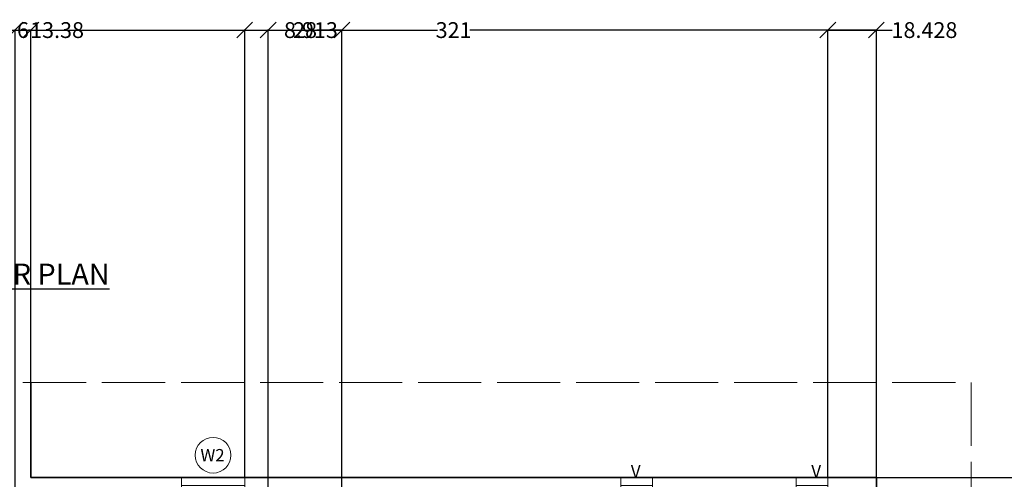
# Model space of a CAD drawing. Units: inches. Extents: x -1198 to -69, y -512 to 437.
# Tile 49 of 50: x -696 to -322, y 263 to 437. Entities that reach past the tile are written whole.
import ezdxf

# ---------------------------------------------------------------- set-up
doc = ezdxf.new("R2010")
doc.units = ezdxf.units.IN
doc.header["$MEASUREMENT"] = 0
doc.linetypes.add('ACAD_ISO02W100', pattern=[15, 12, -3])
for name, color, linetype, lineweight in [('A-ANNO-DIMS', 2, 'Continuous', 18), ('A-ANNO-SYMB', 7, 'Continuous', 18), ('A-ANNO-TEXT', 7, 'Continuous', 25), ('A-WALL', 7, 'Continuous', 35), ('C-PROP', 141, 'ACAD_ISO02W100', 18), ('Doors', 140, 'Continuous', 25), ('windows', 160, 'Continuous', 18)]:
    doc.layers.add(name, color=color, linetype=linetype, lineweight=lineweight)
doc.styles.get("Standard").update_dxf_attribs({"font": 'arial.ttf'})
doc.dimstyles.get("Standard").update_dxf_attribs({"dimtxt": 6, "dimasz": 6, "dimexe": 0.18, "dimexo": 0.0625, "dimgap": 0.09, "dimtad": 0, "dimtih": 1, "dimtoh": 1, "dimdec": 0, "dimzin": 0, "dimdsep": 46, "dimlunit": 4, "dimtxsty": 'Standard', "dimblk": 'OBLIQUE', "dimcen": 0.09, "dimadec": 0, "dimazin": 0, "dimtfac": 1, "dimtdec": 0, "dimtofl": 0, "dimtmove": 0, "dimatfit": 3, "dimfxl": 1, "dimtolj": 1, "dimtzin": 0, "dimarcsym": 0})

# ---------------------------------------------------------------- blocks, each defined once
blk = doc.blocks.new('*U4')
for p, q in [((0, 0), (0, -6)), ((28, 0), (28, -6))]:
    blk.add_line(p, q)
blk.add_lwpolyline([(0, 0), (0, 28), (1.75, 28), (1.75, 0)], close=True)
blk.add_arc((0, 0), 28, 0, 90)
blk = doc.blocks.new('WIN-W2-24')
at = {"ltscale": 10}
for p, q in [((0, 6), (0, 0)), ((24, 6), (24, 0)), ((0, 3), (24, 3))]:
    blk.add_line(p, q, dxfattribs=at)
blk = doc.blocks.new('VENT-12')
at = {"ltscale": 10}
for p, q in [((0, 6), (0, 0)), ((12, 6), (12, 0)), ((0, 3), (12, 3))]:
    blk.add_line(p, q, dxfattribs=at)
blk = doc.blocks.new('TAG-W2')
at = {"ltscale": 10}
blk.add_circle((0, 0), 6.77, dxfattribs=at)
blk.add_text('W2', height=4.7, dxfattribs=at).set_placement((-4.79, -2.36))
blk = doc.blocks.new('_Oblique')
at = {"color": 0, "linetype": 'ByBlock', "lineweight": -2}
blk.add_line((-0.5, -0.5), (0.5, 0.5), dxfattribs=at)
blk = doc.blocks.new('*D63')
at = {"layer": 'A-ANNO-DIMS', "color": 0, "lineweight": -2, "ltscale": 10, "transparency": 16777216}
for p, q in [((-370.69, 263.23), (-79.37, 263.23)), ((-79.55, 263.23), (-79.55, 20.38)), ((-79.55, -228.77), (-79.55, 14.07)), ((-370.69, -228.77), (-79.37, -228.77))]:
    blk.add_line(p, q, dxfattribs=at)
at = {"layer": 'DEFPOINTS', "color": 0, "ltscale": 10, "transparency": 16777216}
for p in [(-370.75, 263.23), (-79.55, 263.23), (-370.75, -228.77)]:
    blk.add_point(p, dxfattribs=at)
at = {"layer": 'A-ANNO-DIMS', "color": 0, "lineweight": -2, "ltscale": 10, "transparency": 16777216, "xscale": 6, "yscale": 6, "zscale": 6}
for p, rotation in [((-79.55, 263.23), 90), ((-79.55, -228.77), 270)]:
    blk.add_blockref('_Oblique', p, dxfattribs=dict(at, rotation=rotation))
at = {"layer": 'A-ANNO-DIMS', "color": 0, "ltscale": 10, "transparency": 16777216, "insert": (-79.55, 17.23), "char_height": 6, "attachment_point": 5}
blk.add_mtext('\\A1;492', dxfattribs=at)
blk = doc.blocks.new('*D64')
at = {"layer": 'A-ANNO-DIMS', "color": 0, "lineweight": -2, "ltscale": 10, "transparency": 16777216}
for p, q in [((-691.75, 299.29), (-691.75, 433.18)), ((-691.75, 433), (-537.39, 433)), ((-370.75, 433), (-525.11, 433)), ((-370.75, 263.29), (-370.75, 433.18))]:
    blk.add_line(p, q, dxfattribs=at)
at = {"layer": 'DEFPOINTS', "color": 0, "ltscale": 10, "transparency": 16777216}
for p in [(-370.75, 433), (-691.75, 299.23), (-370.75, 263.23)]:
    blk.add_point(p, dxfattribs=at)
at = {"layer": 'A-ANNO-DIMS', "color": 0, "lineweight": -2, "ltscale": 10, "transparency": 16777216, "xscale": 6, "yscale": 6, "zscale": 6, "rotation": 180}
blk.add_blockref('_Oblique', (-691.75, 433), dxfattribs=at)
at = {"layer": 'A-ANNO-DIMS', "color": 0, "lineweight": -2, "ltscale": 10, "transparency": 16777216, "xscale": 6, "yscale": 6, "zscale": 6}
blk.add_blockref('_Oblique', (-370.75, 433), dxfattribs=at)
at = {"layer": 'A-ANNO-DIMS', "color": 0, "ltscale": 10, "transparency": 16777216, "insert": (-531.25, 433), "char_height": 6, "attachment_point": 5}
blk.add_mtext('\\A1;321', dxfattribs=at)
blk = doc.blocks.new('*D71')
at = {"layer": 'A-ANNO-DIMS', "color": 0, "lineweight": -2, "ltscale": 10, "transparency": 16777216}
for p, q in [((-601.65, 263.29), (-601.65, 433.18)), ((-601.65, 433), (-592.09, 433)), ((-573.65, 433), (-583.2, 433)), ((-573.65, 263.29), (-573.65, 433.18))]:
    blk.add_line(p, q, dxfattribs=at)
at = {"layer": 'DEFPOINTS', "color": 0, "ltscale": 10, "transparency": 16777216}
for p in [(-573.65, 433), (-601.65, 263.23), (-573.65, 263.23)]:
    blk.add_point(p, dxfattribs=at)
at = {"layer": 'A-ANNO-DIMS', "color": 0, "lineweight": -2, "ltscale": 10, "transparency": 16777216, "xscale": 6, "yscale": 6, "zscale": 6, "rotation": 180}
blk.add_blockref('_Oblique', (-601.65, 433), dxfattribs=at)
at = {"layer": 'A-ANNO-DIMS', "color": 0, "lineweight": -2, "ltscale": 10, "transparency": 16777216, "xscale": 6, "yscale": 6, "zscale": 6}
blk.add_blockref('_Oblique', (-573.65, 433), dxfattribs=at)
at = {"layer": 'A-ANNO-DIMS', "color": 0, "ltscale": 10, "transparency": 16777216, "insert": (-587.65, 433), "char_height": 6, "attachment_point": 5}
blk.add_mtext('\\A1;28', dxfattribs=at)
blk = doc.blocks.new('*D73')
at = {"layer": 'A-ANNO-DIMS', "color": 0, "lineweight": -2, "ltscale": 10, "transparency": 16777216}
for p, q in [((-697.75, 299.29), (-697.75, 433.18)), ((-697.75, 433), (-696.82, 433)), ((-691.75, 433), (-692.68, 433)), ((-691.75, 299.29), (-691.75, 433.18))]:
    blk.add_line(p, q, dxfattribs=at)
at = {"layer": 'DEFPOINTS', "color": 0, "ltscale": 10, "transparency": 16777216}
for p in [(-691.75, 433), (-697.75, 299.23), (-691.75, 299.23)]:
    blk.add_point(p, dxfattribs=at)
at = {"layer": 'A-ANNO-DIMS', "color": 0, "lineweight": -2, "ltscale": 10, "transparency": 16777216, "xscale": 6, "yscale": 6, "zscale": 6, "rotation": 180}
blk.add_blockref('_Oblique', (-697.75, 433), dxfattribs=at)
at = {"layer": 'A-ANNO-DIMS', "color": 0, "lineweight": -2, "ltscale": 10, "transparency": 16777216, "xscale": 6, "yscale": 6, "zscale": 6}
blk.add_blockref('_Oblique', (-691.75, 433), dxfattribs=at)
at = {"layer": 'A-ANNO-DIMS', "color": 0, "ltscale": 10, "transparency": 16777216, "insert": (-694.75, 433), "char_height": 6, "attachment_point": 5}
blk.add_mtext('\\A1;6', dxfattribs=at)
blk = doc.blocks.new('*D76')
at = {"layer": 'A-ANNO-DIMS', "color": 0, "lineweight": -2, "ltscale": 10, "transparency": 16777216}
for p, q in [((-711.13, -38.21), (-711.13, 433.18)), ((-711.13, 433), (-697.75, 433)), ((-697.75, -38.21), (-697.75, 433.18)), ((-697.75, 433), (-691.75, 433))]:
    blk.add_line(p, q, dxfattribs=at)
at = {"layer": 'DEFPOINTS', "color": 0, "ltscale": 10, "transparency": 16777216}
for p in [(-697.75, 433), (-711.13, -38.27), (-697.75, -38.27)]:
    blk.add_point(p, dxfattribs=at)
at = {"layer": 'A-ANNO-DIMS', "color": 0, "lineweight": -2, "ltscale": 10, "transparency": 16777216, "xscale": 6, "yscale": 6, "zscale": 6, "rotation": 180}
blk.add_blockref('_Oblique', (-711.13, 433), dxfattribs=at)
at = {"layer": 'A-ANNO-DIMS', "color": 0, "lineweight": -2, "ltscale": 10, "transparency": 16777216, "xscale": 6, "yscale": 6, "zscale": 6}
blk.add_blockref('_Oblique', (-697.75, 433), dxfattribs=at)
at = {"layer": 'A-ANNO-DIMS', "color": 0, "ltscale": 10, "transparency": 16777216, "insert": (-681.81, 433), "char_height": 6, "attachment_point": 5}
blk.add_mtext('\\A1;13.38', dxfattribs=at)
blk = doc.blocks.new('*D79')
at = {"layer": 'A-ANNO-DIMS', "color": 0, "lineweight": -2, "ltscale": 10, "transparency": 16777216}
for p, q in [((-610.56, 263.29), (-610.56, 433.18)), ((-610.56, 433), (-601.65, 433)), ((-601.65, 263.29), (-601.65, 433.18)), ((-601.65, 433), (-595.65, 433))]:
    blk.add_line(p, q, dxfattribs=at)
at = {"layer": 'DEFPOINTS', "color": 0, "ltscale": 10, "transparency": 16777216}
for p in [(-601.65, 433), (-610.56, 263.23), (-601.65, 263.23)]:
    blk.add_point(p, dxfattribs=at)
at = {"layer": 'A-ANNO-DIMS', "color": 0, "lineweight": -2, "ltscale": 10, "transparency": 16777216, "xscale": 6, "yscale": 6, "zscale": 6, "rotation": 180}
blk.add_blockref('_Oblique', (-610.56, 433), dxfattribs=at)
at = {"layer": 'A-ANNO-DIMS', "color": 0, "lineweight": -2, "ltscale": 10, "transparency": 16777216, "xscale": 6, "yscale": 6, "zscale": 6}
blk.add_blockref('_Oblique', (-601.65, 433), dxfattribs=at)
at = {"layer": 'A-ANNO-DIMS', "color": 0, "ltscale": 10, "transparency": 16777216, "insert": (-585.43, 433), "char_height": 6, "attachment_point": 5}
blk.add_mtext('\\A1;8.913', dxfattribs=at)
blk = doc.blocks.new('*D82')
at = {"layer": 'A-ANNO-DIMS', "color": 0, "lineweight": -2, "ltscale": 10, "transparency": 16777216}
for p, q in [((-389.18, 263.29), (-389.18, 433.18)), ((-389.18, 433), (-370.75, 433)), ((-370.75, 263.29), (-370.75, 433.18)), ((-370.75, 433), (-364.75, 433))]:
    blk.add_line(p, q, dxfattribs=at)
at = {"layer": 'DEFPOINTS', "color": 0, "ltscale": 10, "transparency": 16777216}
for p in [(-370.75, 433), (-389.18, 263.23), (-370.75, 263.23)]:
    blk.add_point(p, dxfattribs=at)
at = {"layer": 'A-ANNO-DIMS', "color": 0, "lineweight": -2, "ltscale": 10, "transparency": 16777216, "xscale": 6, "yscale": 6, "zscale": 6, "rotation": 180}
blk.add_blockref('_Oblique', (-389.18, 433), dxfattribs=at)
at = {"layer": 'A-ANNO-DIMS', "color": 0, "lineweight": -2, "ltscale": 10, "transparency": 16777216, "xscale": 6, "yscale": 6, "zscale": 6}
blk.add_blockref('_Oblique', (-370.75, 433), dxfattribs=at)
at = {"layer": 'A-ANNO-DIMS', "color": 0, "ltscale": 10, "transparency": 16777216, "insert": (-352.48, 433), "char_height": 6, "attachment_point": 5}
blk.add_mtext('\\A1;18.428', dxfattribs=at)

msp = doc.modelspace()

# ---------------------------------------------------------------- linework, layer by layer
at = {"layer": 'A-WALL', "ltscale": 10}
for p, q in [((-691.7509, 299.2277), (-691.7509, 263.2277)), ((-370.7509, 263.2277), (-691.7509, 263.2277)), ((-376.7509, 263.2277), (-691.7509, 263.2277)), ((-370.7509, -228.7723), (-370.7509, 263.2277))]:
    msp.add_line(p, q, dxfattribs=at)
at = {"layer": 'C-PROP', "ltscale": 2}
msp.add_lwpolyline([(-1054.7509, 299.2277), (-334.7509, 299.2277), (-334.7509, -264.7723), (-1054.7509, -264.7723)], close=True, dxfattribs=at)

# ---------------------------------------------------------------- block references
at = {"layer": 'A-ANNO-SYMB'}
msp.add_blockref('TAG-W2', (-622.5812, 271.6962), dxfattribs=at)
at = {"layer": 'Doors', "rotation": 180}
msp.add_blockref('*U4', (-573.6458, 257.2277), dxfattribs=at)
at = {"layer": 'windows'}
msp.add_blockref('WIN-W2-24', (-634.559, 257.228), dxfattribs=at)
at = {"layer": 'windows', "rotation": 180}
for p in [(-455.7361, 263.2273), (-389.1785, 263.2273)]:
    msp.add_blockref('VENT-12', p, dxfattribs=at)

# ---------------------------------------------------------------- texts
at = {"layer": 'A-ANNO-SYMB', "ltscale": 10}
for p in [(-463.9547, 263.2277), (-395.4315, 263.2277)]:
    msp.add_text('V', height=4.6996, dxfattribs=at).set_placement(p)
at = {"layer": 'A-ANNO-TEXT', "ltscale": 10, "insert": (-775.0037, 344.4033), "char_height": 8, "attachment_point": 1}
msp.add_mtext_dynamic_manual_height_columns('{\\fArial|b1|i0|c0|p34;\\LGROUND FLOOR PLAN}', width=340.81761, gutter_width=40, heights=[0], dxfattribs=at)

# ---------------------------------------------------------------- dimensions: what is measured, and where the dimension line sits
at = {"layer": 'A-ANNO-DIMS', "ltscale": 10}
for base, p1, p2, override, picture, middle in [((-697.7509, 433.0036), (-711.1319, -38.2723), (-697.7509, -38.2723), {"dimdec": 2, "dimlfac": 1, "dimrnd": 0, "dimzin": 0, "dimdsep": 46, "dimlunit": 2}, '*D76', (-681.8137, 433.0036)), ((-691.7509, 433.0036), (-697.7509, 299.2277), (-691.7509, 299.2277), {"dimdec": 0, "dimlfac": 1, "dimrnd": 0, "dimzin": 0, "dimdsep": 46, "dimlunit": 2}, '*D73', (-694.7509, 433.0036)), ((-370.7509, 433.0036), (-691.7509, 299.2277), (-370.7509, 263.2277), {"dimdec": 0, "dimlfac": 1, "dimrnd": 0, "dimzin": 0, "dimdsep": 46, "dimlunit": 2}, '*D64', (-531.2509, 433.0036)), ((-601.6458, 433.0036), (-610.5591, 263.2277), (-601.6458, 263.2277), {"dimdec": 3, "dimlfac": 1, "dimrnd": 0, "dimzin": 0, "dimdsep": 46, "dimlunit": 2}, '*D79', (-585.4282, 433.0036)), ((-573.6458, 433.0036), (-601.6458, 263.2277), (-573.6458, 263.2277), {"dimdec": 0, "dimlfac": 1, "dimrnd": 0, "dimzin": 0, "dimdsep": 46, "dimlunit": 2}, '*D71', (-587.6458, 433.0036)), ((-370.7509, 433.0036), (-389.1788, 263.2277), (-370.7509, 263.2277), {"dimdec": 3, "dimlfac": 1, "dimrnd": 0, "dimzin": 0, "dimdsep": 46, "dimlunit": 2}, '*D82', (-352.4828, 433.0036))]:
    dim = msp.add_linear_dim(base=base, p1=p1, p2=p2, dimstyle='Standard', override=override, dxfattribs=at)
    dim.commit()
    dim.dimension.update_dxf_attribs({"geometry": picture, "text_midpoint": middle})
dim = msp.add_linear_dim(base=(-79.5507, 263.2277), p1=(-370.7509, -228.7723), p2=(-370.7509, 263.2277), angle=90, dimstyle='Standard', override={"dimdec": 0, "dimlfac": 1, "dimrnd": 0, "dimzin": 0, "dimdsep": 46, "dimlunit": 2}, dxfattribs=at)
dim.commit()
dim.dimension.update_dxf_attribs({"geometry": '*D63', "text_midpoint": (-79.5507, 17.2277)})

doc.saveas('drawing.dxf')
